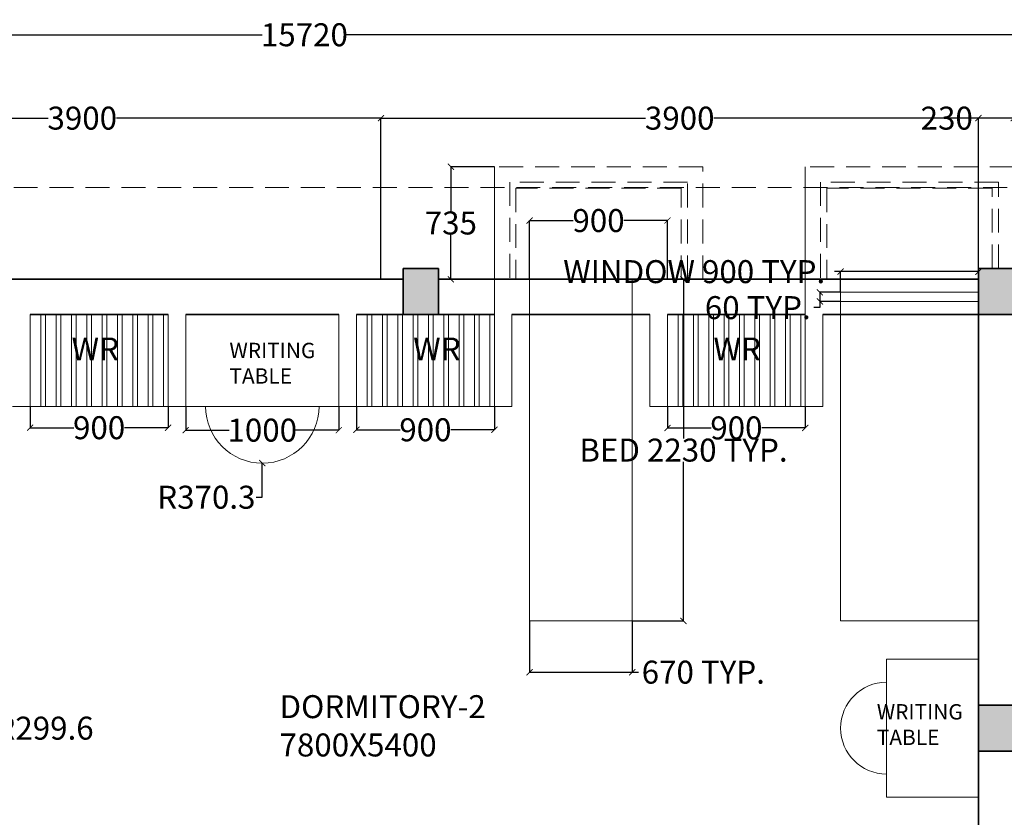
# Model space of a CAD drawing. Units: millimetres. Extents: x 32888 to 53184, y 27889 to 39696.
# Tile 5 of 6: x 41170 to 47598, y 34489 to 39696. Entities that reach past the tile are written whole.
import ezdxf

# ---------------------------------------------------------------- set-up
doc = ezdxf.new("R2010")
doc.units = ezdxf.units.MM
doc.header["$LTSCALE"] = 50
doc.header["$MEASUREMENT"] = 0
doc.linetypes.add('HIDDEN2', pattern=[0.1875, 0.125, -0.0625])
for name, color, linetype, lineweight in [('A-ANNO-DIMS', 2, 'Continuous', 18), ('A-ANNO-TEXT', 7, 'Continuous', 18), ('A-AREA-IDEN', 7, 'Continuous', 18), ('A-COLS', 1, 'Continuous', 35), ('A-COLS-PATT', 18, 'Continuous', 18), ('A-FURN', 8, 'Continuous', 18), ('A-FURN-CASE', 8, 'Continuous', 18), ('A-GLAZ', 4, 'Continuous', 18), ('A-ROOF', 8, 'Continuous', 18), ('A-ROOF-OVHD', 8, 'HIDDEN2', 18), ('A-WALL', 7, 'Continuous', 35)]:
    doc.layers.add(name, color=color, linetype=linetype, lineweight=lineweight)
doc.styles.get("Standard").update_dxf_attribs({"font": 'arial.ttf'})
doc.dimstyles.get("Standard").update_dxf_attribs({"dimtxt": 150, "dimasz": 40, "dimexe": 0.18, "dimexo": 0.0625, "dimgap": 0.09, "dimtad": 0, "dimtih": 1, "dimtoh": 1, "dimdec": 0, "dimzin": 0, "dimdsep": 46, "dimtxsty": 'Standard', "dimblk": 'ARCHTICK', "dimcen": 0, "dimadec": 0, "dimazin": 0, "dimtfac": 1, "dimtdec": 0, "dimtofl": 0, "dimtmove": 0, "dimatfit": 3, "dimldrblk": 'ARCHTICK', "dimfxl": 1, "dimtolj": 1, "dimtzin": 0, "dimarcsym": 1})

# ---------------------------------------------------------------- blocks, each defined once
blk = doc.blocks.new('_ArchTick')
at = {"color": 0, "linetype": 'ByBlock', "const_width": 0.15}
blk.add_lwpolyline([(-0.5, -0.5), (0.5, 0.5)], dxfattribs=at)
blk = doc.blocks.new('*D32')
at = {"layer": 'A-ANNO-DIMS', "color": 0, "lineweight": -2, "ltscale": 50, "transparency": 16777216}
for p, q in [((45398.9, 37170.9), (45398.9, 37030.7)), ((46298.9, 37170.9), (46298.9, 37030.7)), ((45398.9, 37030.9), (45683.4, 37030.9)), ((46298.9, 37030.9), (46014.5, 37030.9))]:
    blk.add_line(p, q, dxfattribs=at)
at = {"layer": 'Defpoints', "color": 0, "ltscale": 50, "transparency": 16777216}
for p in [(45398.9, 37171), (46298.9, 37171), (45398.9, 37030.9)]:
    blk.add_point(p, dxfattribs=at)
at = {"layer": 'A-ANNO-DIMS', "color": 0, "lineweight": -2, "ltscale": 50, "transparency": 16777216, "xscale": 40, "yscale": 40, "zscale": 40, "rotation": 180}
blk.add_blockref('_ArchTick', (45398.9, 37030.9), dxfattribs=at)
at = {"layer": 'A-ANNO-DIMS', "color": 0, "lineweight": -2, "ltscale": 50, "transparency": 16777216, "xscale": 40, "yscale": 40, "zscale": 40}
blk.add_blockref('_ArchTick', (46298.9, 37030.9), dxfattribs=at)
at = {"layer": 'A-ANNO-DIMS', "color": 0, "ltscale": 50, "transparency": 16777216, "insert": (45848.9, 37030.9), "char_height": 150, "attachment_point": 5}
blk.add_mtext('\\A1;900', dxfattribs=at)
blk = doc.blocks.new('*D33')
at = {"layer": 'A-ANNO-DIMS', "color": 0, "lineweight": -2, "ltscale": 50, "transparency": 16777216}
for p, q in [((43368.9, 37170.9), (43368.9, 37018.6)), ((44268.9, 37170.9), (44268.9, 37018.6)), ((43368.9, 37018.8), (43653.4, 37018.8)), ((44268.9, 37018.8), (43984.5, 37018.8))]:
    blk.add_line(p, q, dxfattribs=at)
at = {"layer": 'Defpoints', "color": 0, "ltscale": 50, "transparency": 16777216}
for p in [(43368.9, 37171), (44268.9, 37171), (43368.9, 37018.8)]:
    blk.add_point(p, dxfattribs=at)
at = {"layer": 'A-ANNO-DIMS', "color": 0, "lineweight": -2, "ltscale": 50, "transparency": 16777216, "xscale": 40, "yscale": 40, "zscale": 40, "rotation": 180.0000000000009}
blk.add_blockref('_ArchTick', (43368.9, 37018.8), dxfattribs=at)
at = {"layer": 'A-ANNO-DIMS', "color": 0, "lineweight": -2, "ltscale": 50, "transparency": 16777216, "xscale": 40, "yscale": 40, "zscale": 40}
blk.add_blockref('_ArchTick', (44268.9, 37018.8), dxfattribs=at)
at = {"layer": 'A-ANNO-DIMS', "color": 0, "ltscale": 50, "transparency": 16777216, "insert": (43818.9, 37018.8), "char_height": 150, "attachment_point": 5}
blk.add_mtext('\\A1;900', dxfattribs=at)
blk = doc.blocks.new('*D34')
at = {"layer": 'A-ANNO-DIMS', "color": 0, "lineweight": -2, "ltscale": 50, "transparency": 16777216}
for p, q in [((42253.9, 37170.9), (42253.9, 37016.1)), ((43253.9, 37170.9), (43253.9, 37016.1)), ((42253.9, 37016.3), (42537.2, 37016.3)), ((43253.9, 37016.3), (42970.7, 37016.3))]:
    blk.add_line(p, q, dxfattribs=at)
at = {"layer": 'Defpoints', "color": 0, "ltscale": 50, "transparency": 16777216}
for p in [(42253.9, 37171), (43253.9, 37171), (42253.9, 37016.3)]:
    blk.add_point(p, dxfattribs=at)
at = {"layer": 'A-ANNO-DIMS', "color": 0, "lineweight": -2, "ltscale": 50, "transparency": 16777216, "xscale": 40, "yscale": 40, "zscale": 40}
for p, rotation in [((42253.9, 37016.3), 179.9999999999992), ((43253.9, 37016.3), 359.9999999999992)]:
    blk.add_blockref('_ArchTick', p, dxfattribs=dict(at, rotation=rotation))
at = {"layer": 'A-ANNO-DIMS', "color": 0, "ltscale": 50, "transparency": 16777216, "insert": (42753.9, 37016.3), "char_height": 150, "attachment_point": 5}
blk.add_mtext('\\A1;1000', dxfattribs=at)
blk = doc.blocks.new('*D35')
at = {"layer": 'A-ANNO-DIMS', "color": 0, "lineweight": -2, "ltscale": 50, "transparency": 16777216}
for p, q in [((41238.9, 37170.9), (41238.9, 37032.2)), ((42138.9, 37170.9), (42138.9, 37032.2)), ((41238.9, 37032.3), (41523.4, 37032.3)), ((42138.9, 37032.3), (41854.5, 37032.3))]:
    blk.add_line(p, q, dxfattribs=at)
at = {"layer": 'Defpoints', "color": 0, "ltscale": 50, "transparency": 16777216}
for p in [(41238.9, 37171), (42138.9, 37171), (41238.9, 37032.3)]:
    blk.add_point(p, dxfattribs=at)
at = {"layer": 'A-ANNO-DIMS', "color": 0, "lineweight": -2, "ltscale": 50, "transparency": 16777216, "xscale": 40, "yscale": 40, "zscale": 40}
for p, rotation in [((41238.9, 37032.3), 179.999999999988), ((42138.9, 37032.3), 359.999999999988)]:
    blk.add_blockref('_ArchTick', p, dxfattribs=dict(at, rotation=rotation))
at = {"layer": 'A-ANNO-DIMS', "color": 0, "ltscale": 50, "transparency": 16777216, "insert": (41688.9, 37032.3), "char_height": 150, "attachment_point": 5}
blk.add_mtext('\\A1;900', dxfattribs=at)
blk = doc.blocks.new('*D43')
at = {"layer": 'A-ANNO-DIMS', "color": 0, "lineweight": -2, "ltscale": 50, "transparency": 16777216}
for p, q in [((44268.9, 38736), (43984.7, 38736)), ((43984.9, 38736), (43984.9, 38445.2)), ((43984.9, 38001), (43984.9, 38291.8)), ((44268.9, 38001), (43984.7, 38001))]:
    blk.add_line(p, q, dxfattribs=at)
at = {"layer": 'Defpoints', "color": 0, "ltscale": 50, "transparency": 16777216}
for p in [(43984.9, 38736), (44268.9, 38736), (44268.9, 38001)]:
    blk.add_point(p, dxfattribs=at)
at = {"layer": 'A-ANNO-DIMS', "color": 0, "lineweight": -2, "ltscale": 50, "transparency": 16777216, "xscale": 40, "yscale": 40, "zscale": 40}
for p, rotation in [((43984.9, 38736), 90), ((43984.9, 38001), 270)]:
    blk.add_blockref('_ArchTick', p, dxfattribs=dict(at, rotation=rotation))
at = {"layer": 'A-ANNO-DIMS', "color": 0, "ltscale": 50, "transparency": 16777216, "insert": (43984.9, 38368.5), "char_height": 150, "attachment_point": 5}
blk.add_mtext('\\A1;735', dxfattribs=at)
blk = doc.blocks.new('*D44')
at = {"layer": 'A-ANNO-DIMS', "color": 0, "lineweight": -2, "ltscale": 50, "transparency": 16777216}
for p, q in [((44498.9, 38001.1), (44498.9, 38384.7)), ((44498.9, 38384.5), (44783.4, 38384.5)), ((45398.9, 38384.5), (45114.5, 38384.5)), ((45398.9, 38001.1), (45398.9, 38384.7))]:
    blk.add_line(p, q, dxfattribs=at)
at = {"layer": 'Defpoints', "color": 0, "ltscale": 50, "transparency": 16777216}
for p in [(45398.9, 38384.5), (44498.9, 38001), (45398.9, 38001)]:
    blk.add_point(p, dxfattribs=at)
at = {"layer": 'A-ANNO-DIMS', "color": 0, "lineweight": -2, "ltscale": 50, "transparency": 16777216, "xscale": 40, "yscale": 40, "zscale": 40, "rotation": 180}
blk.add_blockref('_ArchTick', (44498.9, 38384.5), dxfattribs=at)
at = {"layer": 'A-ANNO-DIMS', "color": 0, "lineweight": -2, "ltscale": 50, "transparency": 16777216, "xscale": 40, "yscale": 40, "zscale": 40}
blk.add_blockref('_ArchTick', (45398.9, 38384.5), dxfattribs=at)
at = {"layer": 'A-ANNO-DIMS', "color": 0, "ltscale": 50, "transparency": 16777216, "insert": (44948.9, 38384.5), "char_height": 150, "attachment_point": 5}
blk.add_mtext('\\A1;900', dxfattribs=at)
blk = doc.blocks.new('*D50')
at = {"layer": 'A-ANNO-DIMS', "color": 0, "lineweight": -2, "ltscale": 50, "transparency": 16777216}
for p, q in [((47428.9, 39052.9), (47388.9, 39052.9)), ((47428.9, 38071.1), (47428.9, 39053.1)), ((47658.9, 39052.9), (47428.9, 39052.9)), ((47658.9, 38071.1), (47658.9, 39053.1))]:
    blk.add_line(p, q, dxfattribs=at)
at = {"layer": 'Defpoints', "color": 0, "ltscale": 50, "transparency": 16777216}
for p in [(47428.9, 39052.9), (47428.9, 38071), (47658.9, 38071)]:
    blk.add_point(p, dxfattribs=at)
at = {"layer": 'A-ANNO-DIMS', "color": 0, "lineweight": -2, "ltscale": 50, "transparency": 16777216, "xscale": 40, "yscale": 40, "zscale": 40}
for p, rotation in [((47428.9, 39052.9), 179.9999999999982), ((47658.9, 39052.9), 359.9999999999982)]:
    blk.add_blockref('_ArchTick', p, dxfattribs=dict(at, rotation=rotation))
at = {"layer": 'A-ANNO-DIMS', "color": 0, "ltscale": 50, "transparency": 16777216, "insert": (47222.1, 39052.9), "char_height": 150, "attachment_point": 5}
blk.add_mtext('\\A1;230', dxfattribs=at)
blk = doc.blocks.new('*D51')
at = {"layer": 'A-ANNO-DIMS', "color": 0, "lineweight": -2, "ltscale": 50, "transparency": 16777216}
for p, q in [((43528.9, 38001.1), (43528.9, 39053.1)), ((43528.9, 39052.9), (45255.2, 39052.9)), ((47428.9, 39052.9), (45702.7, 39052.9)), ((47428.9, 38001.1), (47428.9, 39053.1))]:
    blk.add_line(p, q, dxfattribs=at)
at = {"layer": 'Defpoints', "color": 0, "ltscale": 50, "transparency": 16777216}
for p in [(43528.9, 39052.9), (43528.9, 38001), (47428.9, 38001)]:
    blk.add_point(p, dxfattribs=at)
at = {"layer": 'A-ANNO-DIMS', "color": 0, "lineweight": -2, "ltscale": 50, "transparency": 16777216, "xscale": 40, "yscale": 40, "zscale": 40, "rotation": 180}
blk.add_blockref('_ArchTick', (43528.9, 39052.9), dxfattribs=at)
at = {"layer": 'A-ANNO-DIMS', "color": 0, "lineweight": -2, "ltscale": 50, "transparency": 16777216, "xscale": 40, "yscale": 40, "zscale": 40}
blk.add_blockref('_ArchTick', (47428.9, 39052.9), dxfattribs=at)
at = {"layer": 'A-ANNO-DIMS', "color": 0, "ltscale": 50, "transparency": 16777216, "insert": (45478.9, 39052.9), "char_height": 150, "attachment_point": 5}
blk.add_mtext('\\A1;3900', dxfattribs=at)
blk = doc.blocks.new('*D52')
at = {"layer": 'A-ANNO-DIMS', "color": 0, "lineweight": -2, "ltscale": 50, "transparency": 16777216}
for p, q in [((39628.9, 38001.1), (39628.9, 39053.3)), ((39628.9, 39053.1), (41355.2, 39053.1)), ((43528.9, 39053.1), (41802.7, 39053.1)), ((43528.9, 38001.1), (43528.9, 39053.3))]:
    blk.add_line(p, q, dxfattribs=at)
at = {"layer": 'Defpoints', "color": 0, "ltscale": 50, "transparency": 16777216}
for p in [(39628.9, 39053.1), (39628.9, 38001), (43528.9, 38001)]:
    blk.add_point(p, dxfattribs=at)
at = {"layer": 'A-ANNO-DIMS', "color": 0, "lineweight": -2, "ltscale": 50, "transparency": 16777216, "xscale": 40, "yscale": 40, "zscale": 40, "rotation": 180}
blk.add_blockref('_ArchTick', (39628.9, 39053.1), dxfattribs=at)
at = {"layer": 'A-ANNO-DIMS', "color": 0, "lineweight": -2, "ltscale": 50, "transparency": 16777216, "xscale": 40, "yscale": 40, "zscale": 40}
blk.add_blockref('_ArchTick', (43528.9, 39053.1), dxfattribs=at)
at = {"layer": 'A-ANNO-DIMS', "color": 0, "ltscale": 50, "transparency": 16777216, "insert": (41578.9, 39053.1), "char_height": 150, "attachment_point": 5}
blk.add_mtext('\\A1;3900', dxfattribs=at)
blk = doc.blocks.new('*D57')
at = {"layer": 'A-ANNO-DIMS', "color": 0, "lineweight": -2, "ltscale": 50, "transparency": 16777216}
for p, q in [((35168.9, 38001.1), (35168.9, 39597.3)), ((35168.9, 39597.2), (42753.9, 39597.2)), ((50888.9, 39597.2), (43304, 39597.2)), ((50888.9, 38001.1), (50888.9, 39597.3))]:
    blk.add_line(p, q, dxfattribs=at)
at = {"layer": 'Defpoints', "color": 0, "ltscale": 50, "transparency": 16777216}
for p in [(50888.9, 39597.2), (35168.9, 38001), (50888.9, 38001)]:
    blk.add_point(p, dxfattribs=at)
at = {"layer": 'A-ANNO-DIMS', "color": 0, "lineweight": -2, "ltscale": 50, "transparency": 16777216, "xscale": 40, "yscale": 40, "zscale": 40, "rotation": 180}
blk.add_blockref('_ArchTick', (35168.9, 39597.2), dxfattribs=at)
at = {"layer": 'A-ANNO-DIMS', "color": 0, "lineweight": -2, "ltscale": 50, "transparency": 16777216, "xscale": 40, "yscale": 40, "zscale": 40}
blk.add_blockref('_ArchTick', (50888.9, 39597.2), dxfattribs=at)
at = {"layer": 'A-ANNO-DIMS', "color": 0, "ltscale": 50, "transparency": 16777216, "insert": (43028.9, 39597.2), "char_height": 150, "attachment_point": 5}
blk.add_mtext('\\A1;15720', dxfattribs=at)
blk = doc.blocks.new('BED-SINGLE-900')
for p in [(900, 2230), (0, 0)]:
    blk.add_line(p, (900, 0))
blk = doc.blocks.new('BED-NARROW-670')
for p, q in [((0, 2230), (0, 0)), ((670, 2230), (670, 0)), ((0, 0), (670, 0))]:
    blk.add_line(p, q)
blk = doc.blocks.new('DESK-WITH-CHAIR-900')
for p, q in [((0, 299.6), (0, 899.6)), ((900, 899.6), (900, 299.6)), ((900, 299.6), (0, 299.6))]:
    blk.add_line(p, q)
blk.add_arc((450, 299.6), 299.6, 180, 0)
blk = doc.blocks.new('WARDROBE-SLATTED-PANEL-900')
at = {"ltscale": 50}
for p, q in [((-830, 600), (-830, 0)), ((-800, 600), (-800, 0)), ((-730, 600), (-730, 0)), ((-700, 600), (-700, 0)), ((-630, 600), (-630, 0)), ((-600, 600), (-600, 0)), ((-530, 600), (-530, 0)), ((-500, 600), (-500, 0)), ((-430, 600), (-430, 0)), ((-400, 600), (-400, 0)), ((-330, 600), (-330, 0)), ((-300, 600), (-300, 0)), ((-230, 600), (-230, 0)), ((-200, 600), (-200, 0)), ((-130, 600), (-130, 0)), ((-100, 600), (-100, 0)), ((-30, 600), (-30, 0)), ((-30, 0), (0, 0))]:
    blk.add_line(p, q, dxfattribs=at)
blk = doc.blocks.new('WINDOW-900')
for p, q in [((900, 60), (0, 60)), ((900, 0), (0, 0))]:
    blk.add_line(p, q)
blk = doc.blocks.new('COLUMN-IN-WALL-230x300')
for points in [[(0, 300), (230, 300)], [(230, 0), (0, 0)]]:
    blk.add_lwpolyline(points)
blk = doc.blocks.new('COLUMN-EDGE-230x300')
for points in [[(0, 300), (0, 0)], [(230, 0), (230, 300)], [(230, 0), (0, 0)]]:
    blk.add_lwpolyline(points)
blk = doc.blocks.new('*D69')
at = {"layer": 'A-ANNO-DIMS', "color": 0, "lineweight": -2, "ltscale": 50, "transparency": 16777216}
for p, q in [((45169, 38001), (45503.6, 38001)), ((45503.4, 38001), (45503.4, 36962.7)), ((45503.4, 35771), (45503.4, 36809.3)), ((45169, 35771), (45503.6, 35771))]:
    blk.add_line(p, q, dxfattribs=at)
at = {"layer": 'Defpoints', "color": 0, "ltscale": 50, "transparency": 16777216}
for p in [(45168.9, 38001), (45503.4, 38001), (45168.9, 35771)]:
    blk.add_point(p, dxfattribs=at)
at = {"layer": 'A-ANNO-DIMS', "color": 0, "lineweight": -2, "ltscale": 50, "transparency": 16777216, "xscale": 40, "yscale": 40, "zscale": 40}
for p, rotation in [((45503.4, 38001), 90), ((45503.4, 35771), 270)]:
    blk.add_blockref('_ArchTick', p, dxfattribs=dict(at, rotation=rotation))
at = {"layer": 'A-ANNO-DIMS', "color": 0, "ltscale": 50, "transparency": 16777216, "insert": (45503.4, 36886), "char_height": 150, "attachment_point": 5}
blk.add_mtext('\\A1;BED 2230 TYP.', dxfattribs=at)
blk = doc.blocks.new('*D70')
at = {"layer": 'A-ANNO-DIMS', "color": 0, "lineweight": -2, "ltscale": 50, "transparency": 16777216}
for p, q in [((44498.9, 35770.9), (44498.9, 35436.3)), ((45168.9, 35770.9), (45168.9, 35436.3)), ((44498.9, 35436.5), (45168.9, 35436.5)), ((45168.9, 35436.5), (45208.9, 35436.5))]:
    blk.add_line(p, q, dxfattribs=at)
at = {"layer": 'Defpoints', "color": 0, "ltscale": 50, "transparency": 16777216}
for p in [(44498.9, 35771), (45168.9, 35771), (45168.9, 35436.5)]:
    blk.add_point(p, dxfattribs=at)
at = {"layer": 'A-ANNO-DIMS', "color": 0, "lineweight": -2, "ltscale": 50, "transparency": 16777216, "xscale": 40, "yscale": 40, "zscale": 40, "rotation": 180}
blk.add_blockref('_ArchTick', (44498.9, 35436.5), dxfattribs=at)
at = {"layer": 'A-ANNO-DIMS', "color": 0, "lineweight": -2, "ltscale": 50, "transparency": 16777216, "xscale": 40, "yscale": 40, "zscale": 40}
blk.add_blockref('_ArchTick', (45168.9, 35436.5), dxfattribs=at)
at = {"layer": 'A-ANNO-DIMS', "color": 0, "ltscale": 50, "transparency": 16777216, "insert": (45632.8, 35436.5), "char_height": 150, "attachment_point": 5}
blk.add_mtext('\\A1;670 TYP.', dxfattribs=at)
blk = doc.blocks.new('*D71')
at = {"layer": 'A-ANNO-DIMS', "color": 0, "lineweight": -2, "ltscale": 50, "transparency": 16777216}
for p, q in [((46528.9, 38051), (46488.9, 38051)), ((46528.9, 37916.1), (46528.9, 38051.2)), ((47428.9, 38051), (46528.9, 38051)), ((47428.9, 37916.1), (47428.9, 38051.2))]:
    blk.add_line(p, q, dxfattribs=at)
at = {"layer": 'Defpoints', "color": 0, "ltscale": 50, "transparency": 16777216}
for p in [(46528.9, 38051), (46528.9, 37916), (47428.9, 37916)]:
    blk.add_point(p, dxfattribs=at)
at = {"layer": 'A-ANNO-DIMS', "color": 0, "lineweight": -2, "ltscale": 50, "transparency": 16777216, "xscale": 40, "yscale": 40, "zscale": 40, "rotation": 180}
blk.add_blockref('_ArchTick', (46528.9, 38051), dxfattribs=at)
at = {"layer": 'A-ANNO-DIMS', "color": 0, "lineweight": -2, "ltscale": 50, "transparency": 16777216, "xscale": 40, "yscale": 40, "zscale": 40}
blk.add_blockref('_ArchTick', (47428.9, 38051), dxfattribs=at)
at = {"layer": 'A-ANNO-DIMS', "color": 0, "ltscale": 50, "transparency": 16777216, "insert": (45573.6, 38051), "char_height": 150, "attachment_point": 5}
blk.add_mtext('\\A1;WINDOW 900 TYP.', dxfattribs=at)
blk = doc.blocks.new('*D72')
at = {"layer": 'A-ANNO-DIMS', "color": 0, "lineweight": -2, "ltscale": 50, "transparency": 16777216}
for p, q in [((46528.9, 37916), (46393.8, 37916)), ((46393.9, 37916), (46393.9, 37856)), ((46393.9, 37816), (46353.9, 37816)), ((46528.9, 37856), (46393.8, 37856)), ((46393.9, 37856), (46393.9, 37816))]:
    blk.add_line(p, q, dxfattribs=at)
at = {"layer": 'Defpoints', "color": 0, "ltscale": 50, "transparency": 16777216}
for p in [(46528.9, 37916), (46393.9, 37856), (46528.9, 37856)]:
    blk.add_point(p, dxfattribs=at)
at = {"layer": 'A-ANNO-DIMS', "color": 0, "lineweight": -2, "ltscale": 50, "transparency": 16777216, "xscale": 40, "yscale": 40, "zscale": 40}
for p, rotation in [((46393.9, 37916), 90), ((46393.9, 37856), 270)]:
    blk.add_blockref('_ArchTick', p, dxfattribs=dict(at, rotation=rotation))
at = {"layer": 'A-ANNO-DIMS', "color": 0, "ltscale": 50, "transparency": 16777216, "insert": (45988.4, 37816), "char_height": 150, "attachment_point": 5}
blk.add_mtext('\\A1;60 TYP.', dxfattribs=at)
blk = doc.blocks.new('*D77')
at = {"layer": 'A-ANNO-DIMS', "color": 0, "lineweight": -2, "ltscale": 50, "transparency": 16777216}
for p, q in [((50889, 38071), (52833.2, 38071)), ((52833, 38071), (52833, 33982.7)), ((52833, 29741), (52833, 33829.3)), ((43354, 29741), (52833.2, 29741))]:
    blk.add_line(p, q, dxfattribs=at)
at = {"layer": 'Defpoints', "color": 0, "ltscale": 50, "transparency": 16777216}
for p in [(50888.9, 38071), (43353.9, 29741), (52833, 29741)]:
    blk.add_point(p, dxfattribs=at)
at = {"layer": 'A-ANNO-DIMS', "color": 0, "lineweight": -2, "ltscale": 50, "transparency": 16777216, "xscale": 40, "yscale": 40, "zscale": 40}
for p, rotation in [((52833, 38071), 90), ((52833, 29741), 270)]:
    blk.add_blockref('_ArchTick', p, dxfattribs=dict(at, rotation=rotation))
at = {"layer": 'A-ANNO-DIMS', "color": 0, "ltscale": 50, "transparency": 16777216, "insert": (52833, 33906), "char_height": 150, "attachment_point": 5}
blk.add_mtext('\\A1;8330', dxfattribs=at)
blk = doc.blocks.new('*D80')
at = {"layer": 'A-ANNO-DIMS', "color": 0, "lineweight": -2, "ltscale": 50, "transparency": 16777216}
for p, q in [((42753.9, 36578.5), (42753.9, 36800.7)), ((42713.9, 36578.5), (42753.9, 36578.5))]:
    blk.add_line(p, q, dxfattribs=at)
at = {"layer": 'Defpoints', "color": 0, "ltscale": 50, "transparency": 16777216}
for p in [(42753.9, 37171), (42753.9, 36800.7)]:
    blk.add_point(p, dxfattribs=at)
at = {"layer": 'A-ANNO-DIMS', "color": 0, "lineweight": -2, "ltscale": 50, "transparency": 16777216, "xscale": 40, "yscale": 40, "zscale": 40, "rotation": 90}
blk.add_blockref('_ArchTick', (42753.9, 36800.7), dxfattribs=at)
at = {"layer": 'A-ANNO-DIMS', "color": 0, "ltscale": 50, "transparency": 16777216, "insert": (42389, 36578.5), "char_height": 150, "attachment_point": 5}
blk.add_mtext('\\A1;R370.3', dxfattribs=at)
blk = doc.blocks.new('*D81')
at = {"layer": 'A-ANNO-DIMS', "color": 0, "lineweight": -2, "ltscale": 50, "transparency": 16777216}
blk.add_line((40708.3, 35071), (40528.5, 35071), dxfattribs=at)
at = {"layer": 'Defpoints', "color": 0, "ltscale": 50, "transparency": 16777216}
for p in [(40228.9, 35071), (40528.5, 35071)]:
    blk.add_point(p, dxfattribs=at)
at = {"layer": 'A-ANNO-DIMS', "color": 0, "lineweight": -2, "ltscale": 50, "transparency": 16777216, "xscale": 40, "yscale": 40, "zscale": 40, "rotation": 180.0000030600586}
blk.add_blockref('_ArchTick', (40528.5, 35071), dxfattribs=at)
at = {"layer": 'A-ANNO-DIMS', "color": 0, "ltscale": 50, "transparency": 16777216, "insert": (41194.3, 35071), "char_height": 150, "attachment_point": 5}
blk.add_mtext('\\A1;3X R299.6', dxfattribs=at)

msp = doc.modelspace()

# ---------------------------------------------------------------- hatches: boundary and pattern name
at = {"layer": 'A-COLS-PATT', "ltscale": 50}
h = msp.add_hatch(color=256, dxfattribs=at)
h.dxf.hatch_style = 1
h.paths.add_polyline_path([(35398.95, 38071.01), (35168.95, 38071.01), (35168.95, 37771.01), (35398.95, 37771.01)])
h.paths.add_polyline_path([(39628.95, 38071.01), (39398.95, 38071.01), (39398.95, 37771.01), (39628.95, 37771.01)])
h.paths.add_polyline_path([(43903.95, 38071.01), (43673.95, 38071.01), (43673.95, 37771.01), (43903.95, 37771.01)])
h.paths.add_polyline_path([(47658.95, 38071.01), (47428.95, 38071.01), (47428.95, 37771.01), (47658.95, 37771.01)])
h.paths.add_polyline_path([(50888.95, 38071.01), (50658.95, 38071.01), (50658.95, 37771.01), (50888.95, 37771.01)])
h.paths.add_polyline_path([(50888.95, 35221.01), (50658.95, 35221.01), (50658.95, 34921.01), (50888.95, 34921.01)])
h.paths.add_polyline_path([(47658.95, 35221.01), (47428.95, 35221.01), (47428.95, 34921.01), (47658.95, 34921.01)])
h.paths.add_polyline_path([(39628.95, 35071.01), (39628.95, 35221.01), (39398.95, 35221.01), (39398.95, 34921.01), (39628.95, 34921.01)])
h.paths.add_polyline_path([(35398.95, 35221.01), (35168.95, 35221.01), (35168.95, 34921.01), (35398.95, 34921.01)])
h.paths.add_polyline_path([(35398.95, 32371.01), (35168.95, 32371.01), (35168.95, 32071.01), (35398.95, 32071.01)])
h.paths.add_polyline_path([(35418.95, 30571.01), (35168.95, 30571.01), (35168.95, 30271.01), (35418.95, 30271.01)])
h.paths.add_polyline_path([(39642.61, 30571.01), (39392.61, 30571.01), (39392.61, 30271.01), (39642.61, 30271.01)])
h.paths.add_polyline_path([(39628.95, 32371.01), (39398.95, 32371.01), (39398.95, 32071.01), (39628.95, 32071.01)])
h.paths.add_polyline_path([(43903.95, 32371.01), (43673.95, 32371.01), (43673.95, 32071.01), (43903.95, 32071.01)])
h.paths.add_polyline_path([(43903.95, 30571.01), (43653.95, 30571.01), (43653.95, 30271.01), (43903.95, 30271.01)])
h.paths.add_polyline_path([(47658.95, 32441.01), (47428.95, 32441.01), (47428.95, 32141.01), (47658.95, 32141.01)])
h.paths.add_polyline_path([(50888.95, 32414.45), (50658.95, 32414.45), (50658.95, 32114.45), (50888.95, 32114.45)])
h.paths.add_polyline_path([(50888.95, 30571.01), (50638.95, 30571.01), (50638.95, 30271.01), (50888.95, 30271.01)])
h.paths.add_polyline_path([(47678.95, 30571.01), (47428.95, 30571.01), (47428.95, 30341.01), (47678.95, 30341.01)])
h.paths.add_polyline_path([(47678.95, 30341.01), (47428.95, 30341.01), (47428.95, 30271.01), (47678.95, 30271.01)])

# ---------------------------------------------------------------- linework, layer by layer
at = {"layer": 'A-COLS'}
msp.add_lwpolyline([(47658.95, 38071.01), (47428.95, 38071.01)], dxfattribs=at)
at = {"layer": 'A-FURN', "ltscale": 50}
msp.add_arc((42753.95, 37171.01), 370.32, 180, 0, dxfattribs=at)
at = {"layer": 'A-FURN-CASE'}
for p, q in [((41238.95, 37771.01), (41238.95, 37171.01)), ((42138.95, 37171.01), (42138.95, 37771.01)), ((42253.95, 37771.01), (42253.95, 37171.01)), ((43253.95, 37771.01), (43253.95, 37171.01)), ((43368.95, 37771.01), (43368.95, 37171.01)), ((44383.95, 37771.01), (44383.95, 37171.01)), ((45283.95, 37171.01), (45283.95, 37771.01)), ((45398.95, 37771.01), (45398.95, 37171.01)), ((46413.95, 37771.01), (46413.95, 37171.01)), ((44383.95, 37171.01), (41123.95, 37171.01)), ((45398.95, 37171.01), (45283.95, 37171.01)), ((46413.95, 37171.01), (46298.95, 37171.01))]:
    msp.add_line(p, q, dxfattribs=at)
at = {"layer": 'A-FURN-CASE', "ltscale": 50}
msp.add_line((46268.95, 37171.01), (45398.95, 37171.01), dxfattribs=at)
at = {"layer": 'A-ROOF'}
for p, q in [((44268.95, 38736.01), (44268.95, 37171.01)), ((46298.95, 37171.01), (46298.95, 38736.01))]:
    msp.add_line(p, q, dxfattribs=at)
at = {"layer": 'A-ROOF-OVHD', "ltscale": 25}
msp.add_line((34568.95, 38601.01), (51488.95, 38601.01), dxfattribs=at)
for points in [[(45628.95, 38001.01), (45628.95, 38736.01), (44268.95, 38736.01)], [(47658.95, 38736.01), (46298.95, 38736.01)], [(45528.95, 38001.01), (45528.95, 38636.01), (44368.95, 38636.01), (44368.95, 38001.01)], [(47558.95, 38071.01), (47558.95, 38636.01), (46398.95, 38636.01), (46398.95, 38001.01)], [(45488.95, 38001.01), (45488.95, 38596.01), (44408.95, 38596.01), (44408.95, 38001.01)], [(47518.95, 38071.01), (47518.95, 38596.01), (46438.95, 38596.01), (46438.95, 38001.01)]]:
    msp.add_lwpolyline(points, dxfattribs=at)
at = {"layer": 'A-WALL'}
for p, q in [((47428.95, 38071.01), (47428.95, 30271.01)), ((39628.95, 38001.01), (43673.95, 38001.01)), ((43903.95, 38001.01), (47428.95, 38001.01)), ((41238.95, 37771.01), (42138.95, 37771.01)), ((42253.95, 37771.01), (43253.95, 37771.01)), ((43368.95, 37771.01), (44268.95, 37771.01)), ((44383.95, 37771.01), (45283.95, 37771.01)), ((46298.95, 37771.01), (45398.95, 37771.01)), ((46413.95, 37771.01), (49043.95, 37771.01))]:
    msp.add_line(p, q, dxfattribs=at)

# ---------------------------------------------------------------- block references
at = {"layer": 'A-COLS', "rotation": 180}
msp.add_blockref('COLUMN-EDGE-230x300', (43903.95, 38071.01), dxfattribs=at)
at = {"layer": 'A-COLS'}
msp.add_blockref('COLUMN-IN-WALL-230x300', (47428.95, 34921.01), dxfattribs=at)
at = {"layer": 'A-FURN'}
msp.add_blockref('BED-NARROW-670', (44498.95, 35771.01), dxfattribs=at)
at = {"layer": 'A-FURN', "extrusion": (0, 0, -1), "zscale": -1}
msp.add_blockref('BED-SINGLE-900', (-47428.95, 35771.01), dxfattribs=at)
at = {"layer": 'A-FURN', "rotation": 269.9999999999991}
msp.add_blockref('DESK-WITH-CHAIR-900', (46529.37, 35521.01), dxfattribs=at)
at = {"layer": 'A-FURN-CASE'}
for p in [(42138.95, 37171.01), (44268.95, 37171.01), (46298.95, 37171.01)]:
    msp.add_blockref('WARDROBE-SLATTED-PANEL-900', p, dxfattribs=at)
at = {"layer": 'A-GLAZ', "rotation": 180}
msp.add_blockref('WINDOW-900', (47428.95, 37916.01), dxfattribs=at)

# ---------------------------------------------------------------- texts
at = {"layer": 'A-ANNO-TEXT', "ltscale": 50, "attachment_point": 1}
for s, width, insert, char_height in [('WR', 742.516, (41508.95, 37621.01), 150), ('WR', 742.516, (43738.95, 37621.01), 150), ('WR', 742.516, (45698.95, 37621.01), 150), ('WRITING\\PTABLE', 901.3249, (42539.68, 37586.49), 100), ('WRITING\\PTABLE', 901.3249, (46765.7, 35227.71), 100)]:
    msp.add_mtext_dynamic_manual_height_columns(s, width=width, gutter_width=1, heights=[0], dxfattribs=dict(at, insert=insert, char_height=char_height))
at = {"layer": 'A-AREA-IDEN', "ltscale": 50, "insert": (42866.56, 35286.3), "char_height": 150, "attachment_point": 1}
msp.add_mtext_dynamic_manual_height_columns('DORMITORY-2\\P7800X5400', width=901.3249, gutter_width=1, heights=[0], dxfattribs=at)

# ---------------------------------------------------------------- dimensions: what is measured, and where the dimension line sits
at = {"layer": 'A-ANNO-DIMS', "ltscale": 50}
for p1, p2, distance, picture, middle in [((35168.95, 38001.01), (50888.95, 38001.01), 1596.15, '*D57', (43028.95, 39597.16)), ((43528.95, 38001.01), (39628.95, 38001.01), -1052.08, '*D52', (41578.95, 39053.09)), ((47428.95, 38001.01), (43528.95, 38001.01), -1051.9, '*D51', (45478.95, 39052.91)), ((47658.95, 38071.01), (47428.95, 38071.01), -981.9, '*D50', (47222.13, 39052.91)), ((44268.95, 38001.01), (44268.95, 38736.01), 284.05, '*D43', (43984.9, 38368.51)), ((44498.95, 38001.01), (45398.95, 38001.01), 383.47, '*D44', (44948.95, 38384.48)), ((42138.95, 37171.01), (41238.95, 37171.01), 138.66, '*D35', (41688.95, 37032.35)), ((43253.95, 37171.01), (42253.95, 37171.01), 154.76, '*D34', (42753.95, 37016.25)), ((44268.95, 37171.01), (43368.95, 37171.01), 152.23, '*D33', (43818.95, 37018.78)), ((46298.95, 37171.01), (45398.95, 37171.01), 140.14, '*D32', (45848.95, 37030.86))]:
    dim = msp.add_aligned_dim(p1=p1, p2=p2, distance=distance, dimstyle='Standard', override={"dimclrd": 0, "dimclre": 0, "dimclrt": 0}, dxfattribs=at)
    dim.commit()
    dim.dimension.update_dxf_attribs({"geometry": picture, "text_midpoint": middle})
for base, p1, p2, angle, text, picture, middle in [((46528.95, 38051.01), (47428.95, 37916.01), (46528.95, 37916.01), 180, 'WINDOW <> TYP.', '*D71', (45573.61, 38051.01)), ((45503.45, 38001.01), (45168.95, 35771.01), (45168.95, 38001.01), 90, 'BED <> TYP.', '*D69', (45503.45, 36886.01)), ((46393.95, 37856.01), (46528.95, 37916.01), (46528.95, 37856.01), 270, '<> TYP.', '*D72', (45988.38, 37816.01))]:
    dim = msp.add_linear_dim(base=base, p1=p1, p2=p2, angle=angle, text=text, dimstyle='Standard', override={"dimdec": 0, "dimlfac": 1, "dimrnd": 0, "dimzin": 0, "dimdsep": 46, "dimlunit": 2}, dxfattribs=at)
    dim.commit()
    dim.dimension.update_dxf_attribs({"geometry": picture, "text_midpoint": middle})
dim = msp.add_linear_dim(base=(52833.03, 29741.01), p1=(50888.95, 38071.01), p2=(43353.95, 29741.01), angle=90, dimstyle='Standard', override={"dimdec": 0, "dimlfac": 1, "dimrnd": 0, "dimzin": 0, "dimdsep": 46, "dimlunit": 2}, dxfattribs=at)
dim.commit()
dim.dimension.update_dxf_attribs({"geometry": '*D77', "text_midpoint": (52833.03, 33906.01)})
dim = msp.add_radius_dim(center=(42753.95, 37171.01), mpoint=(42753.95, 36800.69), dimstyle='Standard', override={"dimdec": 1, "dimlfac": 1, "dimrnd": 0, "dimzin": 0, "dimdsep": 46, "dimlunit": 2}, dxfattribs=at)
dim.commit()
dim.dimension.update_dxf_attribs({"geometry": '*D80', "text_midpoint": (42389, 36578.5), "dimtype": 164})
dim = msp.add_linear_dim(base=(45168.95, 35436.51), p1=(44498.95, 35771.01), p2=(45168.95, 35771.01), text='<> TYP.', dimstyle='Standard', override={"dimdec": 0, "dimlfac": 1, "dimrnd": 0, "dimzin": 0, "dimdsep": 46, "dimlunit": 2}, dxfattribs=at)
dim.commit()
dim.dimension.update_dxf_attribs({"geometry": '*D70', "text_midpoint": (45632.79, 35436.51)})
dim = msp.add_radius_dim(center=(40228.95, 35071.01), mpoint=(40528.53, 35071.01), text='3X <>', dimstyle='Standard', override={"dimdec": 1, "dimlfac": 1, "dimrnd": 0, "dimzin": 0, "dimdsep": 46, "dimlunit": 2}, dxfattribs=at)
dim.commit()
dim.dimension.update_dxf_attribs({"geometry": '*D81', "text_midpoint": (40708.28, 35071.01), "dimtype": 164})

doc.saveas('drawing.dxf')
